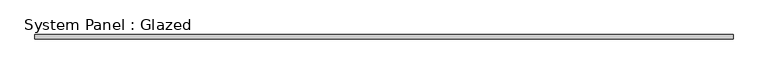
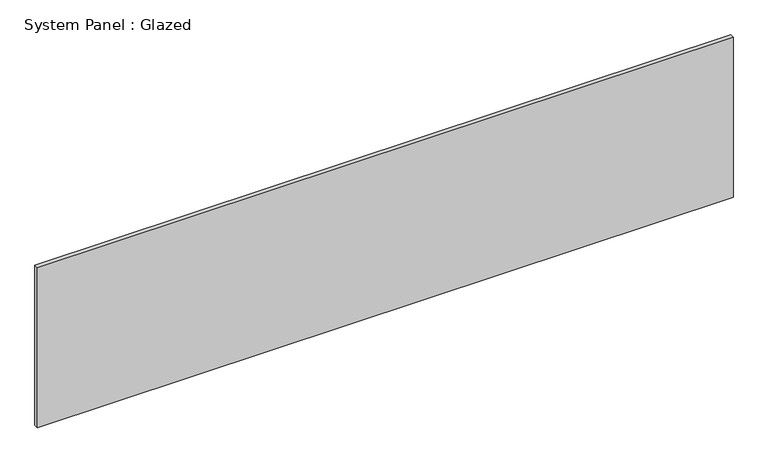
"""IFC4 building model written with IfcOpenShell, lengths in millimetres: plate geometry, System Panel : Glazed."""

from ifc_helpers import new_model, si_unit, origin, origin_with_axes, place, context, project, spatial, polyline, outline, extrude, source, transform, mapped, element, save


def system_panel_glazed_349dd858(model_context):
    return source(origin(), model_context, "Body", "SweptSolid", [
        extrude(outline(polyline([(2057.4, 19.05), (-2057.4, 19.05), (-2057.4, 44.45), (2057.4, 44.45), (2057.4, 19.05)])), origin_with_axes(), (0.0, 0.0, 1.0), 1000.0768654),
    ])


if __name__ == "__main__":
    model = new_model("IFC4")
    model_context = context("Model", 3, world=origin())
    ifc_project = project(units=[si_unit("LENGTHUNIT", "METRE", prefix="MILLI")], contexts=[model_context])
    site = spatial("IfcSite", under=ifc_project)
    building = spatial("IfcBuilding", under=site)
    placement = place(None, origin())
    system_panel_glazed_shape = system_panel_glazed_349dd858(model_context)
    element("IfcPlate", 1, ObjectType="System Panel : Glazed", at=placement, inside=building, context=model_context, shape_type="MappedRepresentation", body=[
        mapped(system_panel_glazed_shape, transform((0.0, 0.0, 0.0), x_axis=(1.0, 0.0, 0.0), y_axis=(0.0, 1.0, 0.0), z_axis=(0.0, 0.0, 1.0))),
    ])
    save(model, "model.ifc")

# Revit data of these elements
# Type "System Panel : Glazed"
#   Construction Type Id = "GSP4R"
#   Analytic Construction = "1/8 in Pilkington single glazing"
#   Visual Light Transmittance = 0.9
#   Solar Heat Gain Coefficient = 0.86
#   Heat Transfer Coefficient (U) = 1.18115 BTU/(h·ft²·°F)
#   Define Thermal Properties by = 1
# Element 1 (IfcPlate, "System Panel : Glazed")
#   Materials on its faces: "Glass"
# Materials
#   "Glass": class "Glass", colour RGB 0 128 192, transparency 0.75, Description = "Soda Lime Glass", Cost = 0
